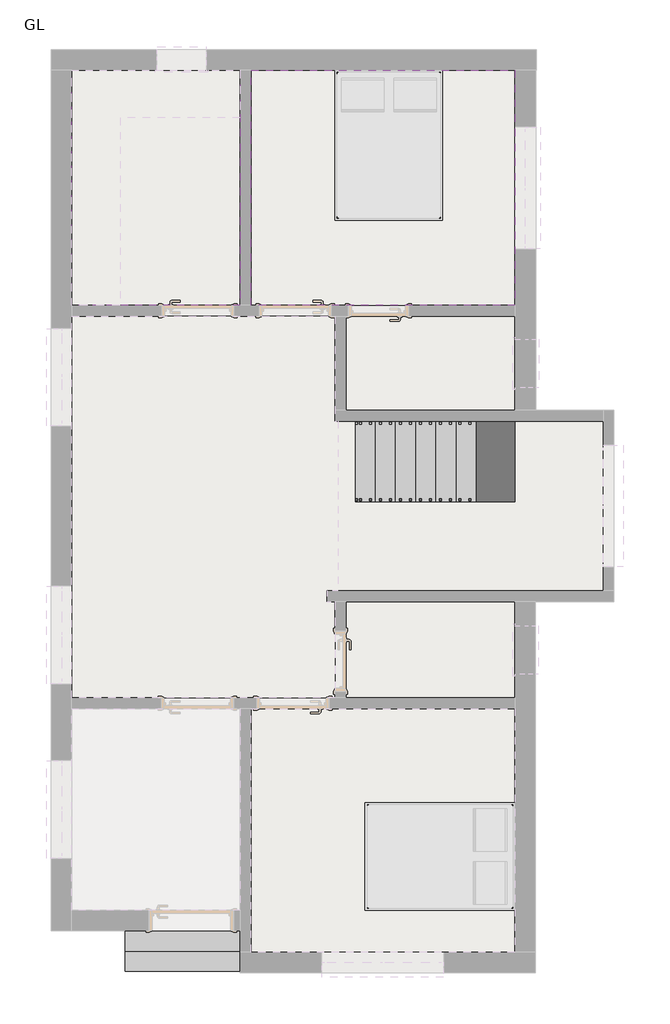
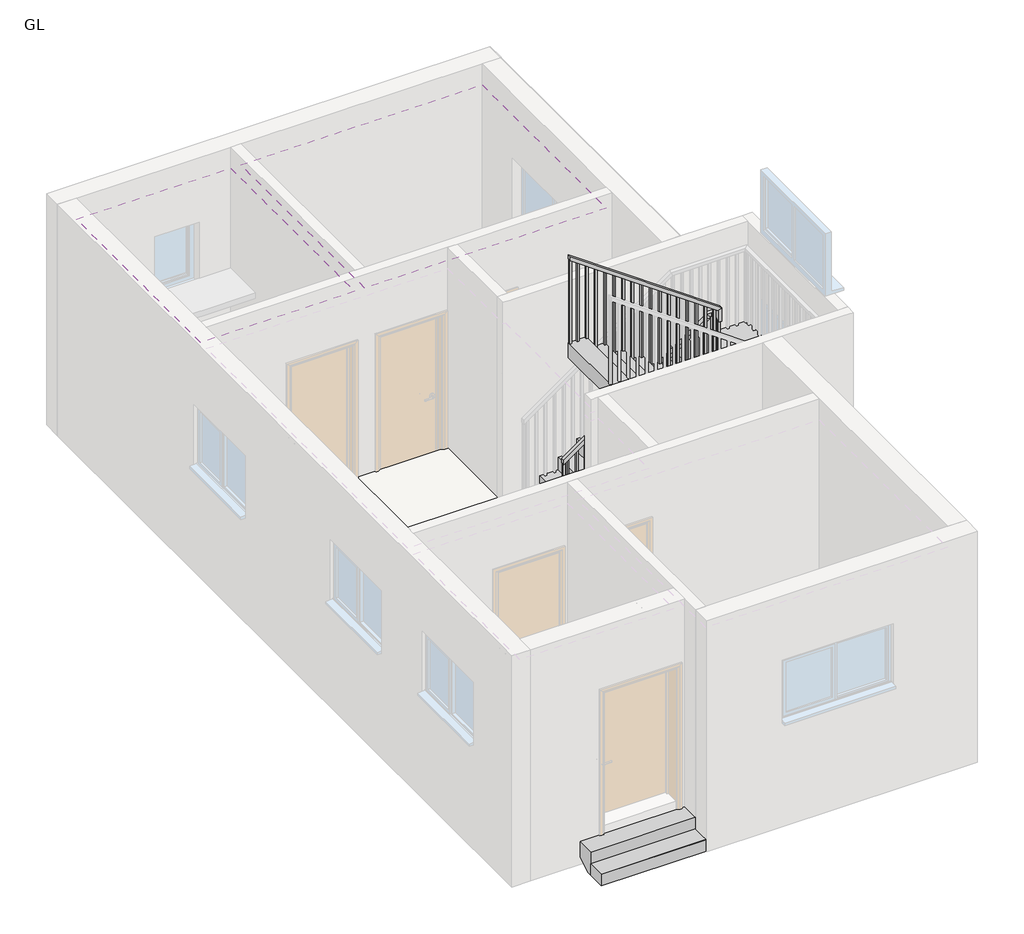
# One storey, part 2 of 3: 4 slabs, 2 coverings, 2 stair flights, 1 railing.
"""IFC4 building model written with IfcOpenShell, lengths in millimetres."""

from ifc_helpers import new_model, si_unit, frame, origin, origin_with_axes, place, context, project, spatial, polyline, outline, extrude, faceted_brep, element, save

model = new_model("IFC4")

# Units and contexts
model_context = context("Model", 3, world=origin())
ifc_project = project(units=[si_unit("LENGTHUNIT", "METRE", prefix="MILLI")], contexts=[model_context])

# Site, building, storey
site = spatial("IfcSite", under=ifc_project)
building = spatial("IfcBuilding", under=site)
storey = spatial("IfcBuildingStorey", under=building, Name="GL", Elevation=0.0)

# Coverings
placement = place(None, origin())
element("IfcCovering", 1, ObjectType="Plain", at=placement, inside=storey, context=model_context, shape_type="SweptSolid", body=[
    extrude(outline(polyline([(-5865.3374044, 11850.4554997), (-3749.5174044, 11850.4554997), (-3749.5174044, 8899.3621562), (-5865.3374044, 8899.3621562), (-5865.3374044, 11850.4554997)])), frame((0.0, 0.0, 2743.2), z_axis=(0.0, 0.0, 1.0), x_axis=(1.0, 0.0, 0.0)), (0.0, 0.0, 1.0), 57.0),
])
element("IfcCovering", 2, ObjectType="Plain", at=placement, inside=storey, context=model_context, shape_type="SweptSolid", body=[
    extrude(outline(polyline([(-3612.3574044, 11850.4554997), (-299.7708818, 11850.4554997), (-299.7708818, 8899.3621562), (-3612.3574044, 8899.3621562), (-3612.3574044, 11850.4554997)])), frame((0.0, 0.0, 2743.2), z_axis=(0.0, 0.0, 1.0), x_axis=(1.0, 0.0, 0.0)), (0.0, 0.0, 1.0), 57.0),
])

# Railing
element("IfcRailing", 3, ObjectType="1100mm", at=placement, inside=storey, context=model_context, shape_type="SolidModel", body=[
    faceted_brep([(-2302.0068409, 6487.2975222, 1279.2941176), (-2302.0068409, 6487.2975222, 1218.028329), (-2302.0068409, 6437.2975222, 1218.028329), (-2302.0068409, 6437.2975222, 1279.2941176), (-350.9568409, 6487.2975222, 2660.8231606), (-300.9568409, 6487.2975222, 2634.9621295), (-300.9568409, 6437.2975222, 2634.9621295), (-350.9568409, 6437.2975222, 2660.8231606), (-350.9568409, 6487.2975222, 2713.6470588), (-300.9568409, 6487.2975222, 2663.6470588), (-300.9568409, 6437.2975222, 2663.6470588), (-350.9568409, 6437.2975222, 2713.6470588), (-225.9568409, 6487.2975222, 2713.6470588), (-225.9568409, 6487.2975222, 2663.6470588), (-275.9568409, 6437.2975222, 2663.6470588), (-275.9568409, 6437.2975222, 2713.6470588), (-225.9568409, 6362.2975222, 2713.6470588), (-225.9568409, 6362.2975222, 2663.6470588), (-275.9568409, 6362.2975222, 2663.6470588), (-275.9568409, 6362.2975222, 2713.6470588), (-225.9568409, 6334.8975222, 2713.6470588), (-275.9568409, 6334.8975222, 2713.6470588), (-275.9568409, 6284.8975222, 2663.6470588), (-225.9568409, 6284.8975222, 2663.6470588)], [[[0, 1, 2, 3]], [[1, 0, 4, 5]], [[2, 1, 5, 6]], [[3, 2, 6, 7]], [[0, 3, 7, 4]], [[5, 4, 8, 9]], [[6, 5, 9, 10]], [[7, 6, 10, 11]], [[4, 7, 11, 8]], [[9, 8, 12, 13]], [[10, 9, 13, 14]], [[11, 10, 14, 15]], [[8, 11, 15, 12]], [[13, 12, 16, 17]], [[14, 13, 17, 18]], [[15, 14, 18, 19]], [[12, 15, 19, 16]], [[20, 21, 22, 23]], [[17, 16, 20, 23]], [[18, 17, 23, 22]], [[19, 18, 22, 21]], [[16, 19, 21, 20]]]),
    faceted_brep([(-225.9568409, 6334.8975222, 2713.6470588), (-225.9568409, 6284.8975222, 2663.6470588), (-275.9568409, 6284.8975222, 2663.6470588), (-275.9568409, 6334.8975222, 2713.6470588), (-225.9568409, 6334.8975222, 2857.2531809), (-275.9568409, 6334.8975222, 2831.3921498), (-275.9568409, 6284.8975222, 2831.3921498), (-225.9568409, 6284.8975222, 2857.2531809)], [[[0, 1, 2, 3]], [[4, 5, 6, 7]], [[1, 0, 4, 7]], [[2, 1, 7, 6]], [[3, 2, 6, 5]], [[0, 3, 5, 4]]]),
    faceted_brep([(-225.9568409, 6284.8975222, 2857.2531809), (-275.9568409, 6284.8975222, 2831.3921498), (-275.9568409, 6334.8975222, 2831.3921498), (-225.9568409, 6334.8975222, 2857.2531809), (-2302.0068409, 6284.8975222, 4327.2941176), (-2302.0068409, 6334.8975222, 4327.2941176), (-2302.0068409, 6334.8975222, 4266.028329), (-2302.0068409, 6284.8975222, 4266.028329)], [[[0, 1, 2, 3]], [[4, 5, 6, 7]], [[1, 0, 4, 7]], [[2, 1, 7, 6]], [[3, 2, 6, 5]], [[0, 3, 5, 4]]]),
    extrude(outline(polyline([(3048.0, -2175.9568409), (4176.7729353, -2175.9568409), (4194.4753141, -2200.9568409), (3048.0, -2200.9568409), (3048.0, -2175.9568409)])), frame((0.0, 6297.3975222, 0.0), z_axis=(0.0, 1.0, 0.0), x_axis=(0.0, 0.0, 1.0)), (0.0, 0.0, 1.0), 25.0),
    extrude(outline(polyline([(3048.0, -2050.9568409), (4088.2610416, -2050.9568409), (4105.9634203, -2075.9568409), (3048.0, -2075.9568409), (3048.0, -2050.9568409)])), frame((0.0, 6297.3975222, 0.0), z_axis=(0.0, 1.0, 0.0), x_axis=(0.0, 0.0, 1.0)), (0.0, 0.0, 1.0), 25.0),
    extrude(outline(polyline([(2868.7058824, -1925.9568409), (3999.7491478, -1925.9568409), (4017.4515265, -1950.9568409), (2868.7058824, -1950.9568409), (2868.7058824, -1925.9568409)])), frame((0.0, 6297.3975222, 0.0), z_axis=(0.0, 1.0, 0.0), x_axis=(0.0, 0.0, 1.0)), (0.0, 0.0, 1.0), 25.0),
    extrude(outline(polyline([(2868.7058824, -1800.9568409), (3911.237254, -1800.9568409), (3928.9396327, -1825.9568409), (2868.7058824, -1825.9568409), (2868.7058824, -1800.9568409)])), frame((0.0, 6297.3975222, 0.0), z_axis=(0.0, 1.0, 0.0), x_axis=(0.0, 0.0, 1.0)), (0.0, 0.0, 1.0), 25.0),
    extrude(outline(polyline([(2689.4117647, -1675.9568409), (3822.7253602, -1675.9568409), (3840.427739, -1700.9568409), (2689.4117647, -1700.9568409), (2689.4117647, -1675.9568409)])), frame((0.0, 6297.3975222, 0.0), z_axis=(0.0, 1.0, 0.0), x_axis=(0.0, 0.0, 1.0)), (0.0, 0.0, 1.0), 25.0),
    extrude(outline(polyline([(2689.4117647, -1550.9568409), (3734.2134664, -1550.9568409), (3751.9158452, -1575.9568409), (2689.4117647, -1575.9568409), (2689.4117647, -1550.9568409)])), frame((0.0, 6297.3975222, 0.0), z_axis=(0.0, 1.0, 0.0), x_axis=(0.0, 0.0, 1.0)), (0.0, 0.0, 1.0), 25.0),
    extrude(outline(polyline([(2510.1176471, -1425.9568409), (3645.7015726, -1425.9568409), (3663.4039514, -1450.9568409), (2510.1176471, -1450.9568409), (2510.1176471, -1425.9568409)])), frame((0.0, 6297.3975222, 0.0), z_axis=(0.0, 1.0, 0.0), x_axis=(0.0, 0.0, 1.0)), (0.0, 0.0, 1.0), 25.0),
    extrude(outline(polyline([(2510.1176471, -1300.9568409), (3557.1896788, -1300.9568409), (3574.8920576, -1325.9568409), (2510.1176471, -1325.9568409), (2510.1176471, -1300.9568409)])), frame((0.0, 6297.3975222, 0.0), z_axis=(0.0, 1.0, 0.0), x_axis=(0.0, 0.0, 1.0)), (0.0, 0.0, 1.0), 25.0),
    extrude(outline(polyline([(2330.8235294, -1175.9568409), (3468.6777851, -1175.9568409), (3486.3801638, -1200.9568409), (2330.8235294, -1200.9568409), (2330.8235294, -1175.9568409)])), frame((0.0, 6297.3975222, 0.0), z_axis=(0.0, 1.0, 0.0), x_axis=(0.0, 0.0, 1.0)), (0.0, 0.0, 1.0), 25.0),
    extrude(outline(polyline([(2330.8235294, -1050.9568409), (3380.1658913, -1050.9568409), (3397.86827, -1075.9568409), (2330.8235294, -1075.9568409), (2330.8235294, -1050.9568409)])), frame((0.0, 6297.3975222, 0.0), z_axis=(0.0, 1.0, 0.0), x_axis=(0.0, 0.0, 1.0)), (0.0, 0.0, 1.0), 25.0),
    extrude(outline(polyline([(2151.5294118, -925.9568409), (3291.6539975, -925.9568409), (3309.3563762, -950.9568409), (2151.5294118, -950.9568409), (2151.5294118, -925.9568409)])), frame((0.0, 6297.3975222, 0.0), z_axis=(0.0, 1.0, 0.0), x_axis=(0.0, 0.0, 1.0)), (0.0, 0.0, 1.0), 25.0),
    extrude(outline(polyline([(2151.5294118, -800.9568409), (3203.1421037, -800.9568409), (3220.8444825, -825.9568409), (2151.5294118, -825.9568409), (2151.5294118, -800.9568409)])), frame((0.0, 6297.3975222, 0.0), z_axis=(0.0, 1.0, 0.0), x_axis=(0.0, 0.0, 1.0)), (0.0, 0.0, 1.0), 25.0),
    extrude(outline(polyline([(1972.2352941, -675.9568409), (3114.6302099, -675.9568409), (3132.3325887, -700.9568409), (1972.2352941, -700.9568409), (1972.2352941, -675.9568409)])), frame((0.0, 6297.3975222, 0.0), z_axis=(0.0, 1.0, 0.0), x_axis=(0.0, 0.0, 1.0)), (0.0, 0.0, 1.0), 25.0),
    extrude(outline(polyline([(1972.2352941, -550.9568409), (3026.1183161, -550.9568409), (3043.8206949, -575.9568409), (1972.2352941, -575.9568409), (1972.2352941, -550.9568409)])), frame((0.0, 6297.3975222, 0.0), z_axis=(0.0, 1.0, 0.0), x_axis=(0.0, 0.0, 1.0)), (0.0, 0.0, 1.0), 25.0),
    extrude(outline(polyline([(1792.9411765, -425.9568409), (2937.6064223, -425.9568409), (2955.3088011, -450.9568409), (1792.9411765, -450.9568409), (1792.9411765, -425.9568409)])), frame((0.0, 6297.3975222, 0.0), z_axis=(0.0, 1.0, 0.0), x_axis=(0.0, 0.0, 1.0)), (0.0, 0.0, 1.0), 25.0),
    extrude(outline(polyline([(1792.9411765, -300.9568409), (2849.0945286, -300.9568409), (2866.7969073, -325.9568409), (1792.9411765, -325.9568409), (1792.9411765, -300.9568409)])), frame((0.0, 6297.3975222, 0.0), z_axis=(0.0, 1.0, 0.0), x_axis=(0.0, 0.0, 1.0)), (0.0, 0.0, 1.0), 25.0),
    extrude(outline(polyline([(-263.4568409, 6412.2975222), (-238.4568409, 6412.2975222), (-238.4568409, 6387.2975222), (-263.4568409, 6387.2975222), (-263.4568409, 6412.2975222)])), frame((0.0, 0.0, 1613.6470588), z_axis=(0.0, 0.0, 1.0), x_axis=(1.0, 0.0, 0.0)), (0.0, 0.0, 1.0), 1050.0),
    extrude(outline(polyline([(2581.1114933, -377.0068409), (1434.3529412, -377.0068409), (1434.3529412, -352.0068409), (2598.8138721, -352.0068409), (2581.1114933, -377.0068409)])), frame((0.0, 6449.7975222, 0.0), z_axis=(0.0, 1.0, 0.0), x_axis=(0.0, 0.0, 1.0)), (0.0, 0.0, 1.0), 25.0),
    extrude(outline(polyline([(2492.5995995, -502.0068409), (1434.3529412, -502.0068409), (1434.3529412, -477.0068409), (2510.3019783, -477.0068409), (2492.5995995, -502.0068409)])), frame((0.0, 6449.7975222, 0.0), z_axis=(0.0, 1.0, 0.0), x_axis=(0.0, 0.0, 1.0)), (0.0, 0.0, 1.0), 25.0),
    extrude(outline(polyline([(2404.0877058, -627.0068409), (1255.0588235, -627.0068409), (1255.0588235, -602.0068409), (2421.7900845, -602.0068409), (2404.0877058, -627.0068409)])), frame((0.0, 6449.7975222, 0.0), z_axis=(0.0, 1.0, 0.0), x_axis=(0.0, 0.0, 1.0)), (0.0, 0.0, 1.0), 25.0),
    extrude(outline(polyline([(2315.575812, -752.0068409), (1255.0588235, -752.0068409), (1255.0588235, -727.0068409), (2333.2781907, -727.0068409), (2315.575812, -752.0068409)])), frame((0.0, 6449.7975222, 0.0), z_axis=(0.0, 1.0, 0.0), x_axis=(0.0, 0.0, 1.0)), (0.0, 0.0, 1.0), 25.0),
    extrude(outline(polyline([(2227.0639182, -877.0068409), (1075.7647059, -877.0068409), (1075.7647059, -852.0068409), (2244.7662969, -852.0068409), (2227.0639182, -877.0068409)])), frame((0.0, 6449.7975222, 0.0), z_axis=(0.0, 1.0, 0.0), x_axis=(0.0, 0.0, 1.0)), (0.0, 0.0, 1.0), 25.0),
    extrude(outline(polyline([(2138.5520244, -1002.0068409), (1075.7647059, -1002.0068409), (1075.7647059, -977.0068409), (2156.2544032, -977.0068409), (2138.5520244, -1002.0068409)])), frame((0.0, 6449.7975222, 0.0), z_axis=(0.0, 1.0, 0.0), x_axis=(0.0, 0.0, 1.0)), (0.0, 0.0, 1.0), 25.0),
    extrude(outline(polyline([(2050.0401306, -1127.0068409), (896.4705882, -1127.0068409), (896.4705882, -1102.0068409), (2067.7425094, -1102.0068409), (2050.0401306, -1127.0068409)])), frame((0.0, 6449.7975222, 0.0), z_axis=(0.0, 1.0, 0.0), x_axis=(0.0, 0.0, 1.0)), (0.0, 0.0, 1.0), 25.0),
    extrude(outline(polyline([(1961.5282368, -1252.0068409), (896.4705882, -1252.0068409), (896.4705882, -1227.0068409), (1979.2306156, -1227.0068409), (1961.5282368, -1252.0068409)])), frame((0.0, 6449.7975222, 0.0), z_axis=(0.0, 1.0, 0.0), x_axis=(0.0, 0.0, 1.0)), (0.0, 0.0, 1.0), 25.0),
    extrude(outline(polyline([(1873.016343, -1377.0068409), (717.1764706, -1377.0068409), (717.1764706, -1352.0068409), (1890.7187218, -1352.0068409), (1873.016343, -1377.0068409)])), frame((0.0, 6449.7975222, 0.0), z_axis=(0.0, 1.0, 0.0), x_axis=(0.0, 0.0, 1.0)), (0.0, 0.0, 1.0), 25.0),
    extrude(outline(polyline([(1784.5044493, -1502.0068409), (717.1764706, -1502.0068409), (717.1764706, -1477.0068409), (1802.206828, -1477.0068409), (1784.5044493, -1502.0068409)])), frame((0.0, 6449.7975222, 0.0), z_axis=(0.0, 1.0, 0.0), x_axis=(0.0, 0.0, 1.0)), (0.0, 0.0, 1.0), 25.0),
    extrude(outline(polyline([(1695.9925555, -1627.0068409), (537.8823529, -1627.0068409), (537.8823529, -1602.0068409), (1713.6949342, -1602.0068409), (1695.9925555, -1627.0068409)])), frame((0.0, 6449.7975222, 0.0), z_axis=(0.0, 1.0, 0.0), x_axis=(0.0, 0.0, 1.0)), (0.0, 0.0, 1.0), 25.0),
    extrude(outline(polyline([(1607.4806617, -1752.0068409), (537.8823529, -1752.0068409), (537.8823529, -1727.0068409), (1625.1830404, -1727.0068409), (1607.4806617, -1752.0068409)])), frame((0.0, 6449.7975222, 0.0), z_axis=(0.0, 1.0, 0.0), x_axis=(0.0, 0.0, 1.0)), (0.0, 0.0, 1.0), 25.0),
    extrude(outline(polyline([(1518.9687679, -1877.0068409), (358.5882353, -1877.0068409), (358.5882353, -1852.0068409), (1536.6711467, -1852.0068409), (1518.9687679, -1877.0068409)])), frame((0.0, 6449.7975222, 0.0), z_axis=(0.0, 1.0, 0.0), x_axis=(0.0, 0.0, 1.0)), (0.0, 0.0, 1.0), 25.0),
    extrude(outline(polyline([(1430.4568741, -2002.0068409), (358.5882353, -2002.0068409), (358.5882353, -1977.0068409), (1448.1592529, -1977.0068409), (1430.4568741, -2002.0068409)])), frame((0.0, 6449.7975222, 0.0), z_axis=(0.0, 1.0, 0.0), x_axis=(0.0, 0.0, 1.0)), (0.0, 0.0, 1.0), 25.0),
    extrude(outline(polyline([(1341.9449803, -2127.0068409), (179.2941176, -2127.0068409), (179.2941176, -2102.0068409), (1359.6473591, -2102.0068409), (1341.9449803, -2127.0068409)])), frame((0.0, 6449.7975222, 0.0), z_axis=(0.0, 1.0, 0.0), x_axis=(0.0, 0.0, 1.0)), (0.0, 0.0, 1.0), 25.0),
    extrude(outline(polyline([(1253.4330865, -2252.0068409), (179.2941176, -2252.0068409), (179.2941176, -2227.0068409), (1271.1354653, -2227.0068409), (1253.4330865, -2252.0068409)])), frame((0.0, 6449.7975222, 0.0), z_axis=(0.0, 1.0, 0.0), x_axis=(0.0, 0.0, 1.0)), (0.0, 0.0, 1.0), 25.0),
    extrude(outline(polyline([(-263.4568409, 6322.3975222), (-238.4568409, 6322.3975222), (-238.4568409, 6297.3975222), (-263.4568409, 6297.3975222), (-263.4568409, 6322.3975222)])), frame((0.0, 0.0, 1613.6470588), z_axis=(0.0, 0.0, 1.0), x_axis=(1.0, 0.0, 0.0)), (0.0, 0.0, 1.0), 1050.0),
    extrude(outline(polyline([(-263.4568409, 6449.7975222), (-263.4568409, 6474.7975222), (-238.4568409, 6474.7975222), (-238.4568409, 6449.7975222), (-263.4568409, 6449.7975222)])), frame((0.0, 0.0, 1613.6470588), z_axis=(0.0, 0.0, 1.0), x_axis=(1.0, 0.0, 0.0)), (0.0, 0.0, 1.0), 1050.0),
    extrude(outline(polyline([(3048.0, -2277.0068409), (4248.3259503, -2277.0068409), (4266.028329, -2302.0068409), (3048.0, -2302.0068409), (3048.0, -2277.0068409)])), frame((0.0, 6297.3975222, 0.0), z_axis=(0.0, 1.0, 0.0), x_axis=(0.0, 0.0, 1.0)), (0.0, 0.0, 1.0), 25.0),
    extrude(outline(polyline([(1218.028329, -2302.0068409), (179.2941176, -2302.0068409), (179.2941176, -2277.0068409), (1235.7307078, -2277.0068409), (1218.028329, -2302.0068409)])), frame((0.0, 6449.7975222, 0.0), z_axis=(0.0, 1.0, 0.0), x_axis=(0.0, 0.0, 1.0)), (0.0, 0.0, 1.0), 25.0),
])

# Slabs
element("IfcSlab", 4, ObjectType="BEDROOM FLOOR", at=placement, inside=storey, context=model_context, shape_type="SweptSolid", body=[
    extrude(outline(polyline([(-299.7708818, 11850.4554997), (-299.7708818, 8899.3621562), (-3612.3574044, 8899.3621562), (-3612.3574044, 11850.4554997), (-299.7708818, 11850.4554997)])), origin_with_axes(), (0.0, 0.0, 1.0), 149.9616),
    extrude(outline(polyline([(-301.4674044, 3840.8703577), (-301.4674044, 786.2154997), (-3617.4374044, 786.2154997), (-3617.4374044, 3840.8703577), (-301.4674044, 3840.8703577)])), origin_with_axes(), (0.0, 0.0, 1.0), 149.9616),
])
element("IfcSlab", 5, ObjectType="HALL FLOOR", at=placement, inside=storey, context=model_context, shape_type="SweptSolid", body=[
    extrude(outline(polyline([(-2558.2574044, 8762.2021562), (-2558.2574044, 7446.2287671), (804.5291182, 7446.2287671), (804.5291182, 5317.8803577), (-2560.7974044, 5317.8803577), (-2560.7974044, 3978.0303577), (-5865.3374044, 3978.0303577), (-5865.3374044, 8762.2021562), (-2558.2574044, 8762.2021562)])), origin_with_axes(), (0.0, 0.0, 1.0), 149.9616),
])
element("IfcSlab", 6, ObjectType="KITCHEN FLOOR", at=placement, inside=storey, context=model_context, shape_type="SweptSolid", body=[
    extrude(outline(polyline([(-3749.5174044, 11850.4554997), (-3749.5174044, 8899.3621562), (-5865.3374044, 8899.3621562), (-5865.3374044, 11850.4554997), (-3749.5174044, 11850.4554997)])), origin_with_axes(), (0.0, 0.0, 1.0), 149.9616),
])
element("IfcSlab", 7, ObjectType="TOILET", at=placement, inside=storey, context=model_context, shape_type="SweptSolid", body=[
    extrude(outline(polyline([(-2423.6374044, 3978.0303577), (-2423.6374044, 5180.7203577), (-301.4674044, 5180.7203577), (-301.4674044, 3978.0303577), (-2423.6374044, 3978.0303577)])), origin_with_axes(), (0.0, 0.0, 1.0), 149.9616),
    extrude(outline(polyline([(-2421.0974044, 7583.3887671), (-2421.0974044, 8762.2021562), (-299.7708818, 8762.2021562), (-299.7708818, 7583.3887671), (-2421.0974044, 7583.3887671)])), origin_with_axes(), (0.0, 0.0, 1.0), 149.9616),
])

# Stair flights
element("IfcStairFlight", 8, ObjectType="1mm_Tread-175mm_Depth", at=placement, inside=storey, context=model_context, shape_type="SolidModel", body=[
    faceted_brep([(-2054.3568409, 7446.2287671, 178.2941176), (-2302.0068409, 7446.2287671, 178.2941176), (-2302.0068409, 6436.8975222, 178.2941176), (-2054.3568409, 6436.8975222, 178.2941176), (-2054.3568409, 7446.2287671, 3.2941176), (-2302.0068409, 7446.2287671, 3.2941176), (-2302.0068409, 6436.8975222, 3.2941176), (-2054.3568409, 6436.8975222, 3.2941176), (-2054.3568409, 7446.2287671, 357.5882353), (-2054.3568409, 6436.8975222, 357.5882353), (-1998.8139986, 6436.8975222, 357.5882353), (-1800.3568409, 6436.8975222, 357.5882353), (-1800.3568409, 7446.2287671, 357.5882353), (-1998.8139986, 7446.2287671, 357.5882353), (-1800.3568409, 7446.2287671, 143.381523), (-1998.8139986, 7446.2287671, 3.2941176), (-1998.8139986, 6436.8975222, 3.2941176), (-1800.3568409, 6436.8975222, 143.381523), (-1546.3568409, 7446.2287671, 536.8823529), (-1800.3568409, 7446.2287671, 536.8823529), (-1800.3568409, 6436.8975222, 536.8823529), (-1546.3568409, 6436.8975222, 536.8823529), (-1546.3568409, 7446.2287671, 322.6756407), (-1546.3568409, 6436.8975222, 322.6756407), (-1292.3568409, 7446.2287671, 716.1764706), (-1546.3568409, 7446.2287671, 716.1764706), (-1546.3568409, 6436.8975222, 716.1764706), (-1292.3568409, 6436.8975222, 716.1764706), (-1292.3568409, 7446.2287671, 501.9697583), (-1292.3568409, 6436.8975222, 501.9697583), (-1038.3568409, 7446.2287671, 895.4705882), (-1292.3568409, 7446.2287671, 895.4705882), (-1292.3568409, 6436.8975222, 895.4705882), (-1038.3568409, 6436.8975222, 895.4705882), (-1038.3568409, 7446.2287671, 681.263876), (-1038.3568409, 6436.8975222, 681.263876), (-784.3568409, 7446.2287671, 1074.7647059), (-1038.3568409, 7446.2287671, 1074.7647059), (-1038.3568409, 6436.8975222, 1074.7647059), (-784.3568409, 6436.8975222, 1074.7647059), (-784.3568409, 7446.2287671, 860.5579936), (-784.3568409, 6436.8975222, 860.5579936), (-530.3568409, 7446.2287671, 1254.0588235), (-784.3568409, 7446.2287671, 1254.0588235), (-784.3568409, 6436.8975222, 1254.0588235), (-530.3568409, 6436.8975222, 1254.0588235), (-530.3568409, 7446.2287671, 1039.8521113), (-530.3568409, 6436.8975222, 1039.8521113), (-276.3568409, 7446.2287671, 1433.3529412), (-530.3568409, 7446.2287671, 1433.3529412), (-530.3568409, 6436.8975222, 1433.3529412), (-276.3568409, 6436.8975222, 1433.3529412), (-276.3568409, 7446.2287671, 1219.1462289), (33.1860014, 6436.8975222, 1437.6470588), (-276.3568409, 6436.8975222, 1437.6470588), (-276.3568409, 5317.8803577, 1612.6470588), (788.0478774, 5317.8803577, 1612.6470588), (788.0478774, 7446.2287671, 1612.6470588), (33.1860014, 7446.2287671, 1612.6470588), (-276.3568409, 7446.2287671, 1612.6470588), (-276.3568409, 6436.8975222, 1612.6470588), (-276.3568409, 6335.2975222, 1612.6470588), (-276.3568409, 5317.8803577, 1437.6470588), (788.0478774, 5317.8803577, 1437.6470588), (788.0478774, 7446.2287671, 1437.6470588), (33.1860014, 7446.2287671, 1437.6470588), (-276.3568409, 6335.2975222, 1437.6470588), (-276.3568409, 5317.8803577, 1791.9411765), (-276.3568409, 6335.2975222, 1791.9411765), (-331.8996832, 6335.2975222, 1791.9411765), (-536.5621226, 6335.2975222, 1791.9411765), (-536.5621226, 5317.8803577, 1791.9411765), (-331.8996832, 5317.8803577, 1791.9411765), (-536.5621226, 5317.8803577, 1582.1146631), (-331.8996832, 5317.8803577, 1437.6470588), (-331.8996832, 6335.2975222, 1437.6470588), (-536.5621226, 6335.2975222, 1582.1146631), (-790.5621226, 5317.8803577, 1971.2352941), (-536.5621226, 5317.8803577, 1971.2352941), (-536.5621226, 6335.2975222, 1971.2352941), (-790.5621226, 6335.2975222, 1971.2352941), (-790.5621226, 5317.8803577, 1761.4087807), (-790.5621226, 6335.2975222, 1761.4087807), (-1044.5621226, 5317.8803577, 2150.5294118), (-790.5621226, 5317.8803577, 2150.5294118), (-790.5621226, 6335.2975222, 2150.5294118), (-1044.5621226, 6335.2975222, 2150.5294118), (-1044.5621226, 5317.8803577, 1940.7028984), (-1044.5621226, 6335.2975222, 1940.7028984), (-1289.1818409, 5317.8803577, 2329.8235294), (-1044.5621226, 5317.8803577, 2329.8235294), (-1044.5621226, 6335.2975222, 2329.8235294), (-1289.1818409, 6335.2975222, 2329.8235294), (-1289.1818409, 5317.8803577, 2113.3756407), (-1289.1818409, 6335.2975222, 2113.3756407), (-1546.3568409, 5317.8803577, 2509.1176471), (-1289.1818409, 5317.8803577, 2509.1176471), (-1289.1818409, 6335.2975222, 2509.1176471), (-1546.3568409, 6335.2975222, 2509.1176471), (-1546.3568409, 5317.8803577, 2294.9109348), (-1546.3568409, 6335.2975222, 2294.9109348), (-1800.3568409, 5317.8803577, 2688.4117647), (-1546.3568409, 5317.8803577, 2688.4117647), (-1546.3568409, 6335.2975222, 2688.4117647), (-1800.3568409, 6335.2975222, 2688.4117647), (-1800.3568409, 5317.8803577, 2474.2050525), (-1800.3568409, 6335.2975222, 2474.2050525), (-2054.3568409, 5317.8803577, 2867.7058824), (-1800.3568409, 5317.8803577, 2867.7058824), (-1800.3568409, 6335.2975222, 2867.7058824), (-2054.3568409, 6335.2975222, 2867.7058824), (-2054.3568409, 5317.8803577, 2653.4991701), (-2054.3568409, 6335.2975222, 2653.4991701), (-2302.0068409, 5317.8803577, 3047.0), (-2054.3568409, 5317.8803577, 3047.0), (-2054.3568409, 6335.2975222, 3047.0), (-2302.0068409, 6335.2975222, 3047.0), (-2302.0068409, 5317.8803577, 2828.3109348), (-2302.0068409, 6335.2975222, 2828.3109348)], [[[0, 1, 2, 3]], [[1, 0, 4, 5]], [[2, 1, 5, 6]], [[3, 2, 6, 7]], [[8, 9, 10, 11, 12, 13]], [[0, 8, 13, 12, 14, 15, 4]], [[0, 3, 9, 8]], [[9, 3, 7, 16, 17, 11, 10]], [[18, 19, 20, 21]], [[19, 18, 22, 14, 12]], [[12, 11, 20, 19]], [[21, 20, 11, 17, 23]], [[24, 25, 26, 27]], [[25, 24, 28, 22, 18]], [[18, 21, 26, 25]], [[27, 26, 21, 23, 29]], [[30, 31, 32, 33]], [[31, 30, 34, 28, 24]], [[24, 27, 32, 31]], [[33, 32, 27, 29, 35]], [[36, 37, 38, 39]], [[37, 36, 40, 34, 30]], [[30, 33, 38, 37]], [[39, 38, 33, 35, 41]], [[42, 43, 44, 45]], [[43, 42, 46, 40, 36]], [[36, 39, 44, 43]], [[45, 44, 39, 41, 47]], [[48, 49, 50, 51]], [[49, 48, 52, 46, 42]], [[42, 45, 50, 49]], [[51, 50, 45, 47, 53, 54]], [[55, 56, 57, 58, 59, 60, 61]], [[56, 55, 62, 63]], [[57, 56, 63, 64]], [[48, 59, 58, 57, 64, 65, 52]], [[48, 51, 54, 60, 59]], [[61, 60, 54, 66]], [[67, 68, 69, 70, 71, 72]], [[55, 67, 72, 71, 73, 74, 62]], [[55, 61, 68, 67]], [[68, 61, 66, 75, 76, 70, 69]], [[77, 78, 79, 80]], [[78, 77, 81, 73, 71]], [[71, 70, 79, 78]], [[80, 79, 70, 76, 82]], [[83, 84, 85, 86]], [[84, 83, 87, 81, 77]], [[77, 80, 85, 84]], [[86, 85, 80, 82, 88]], [[89, 90, 91, 92]], [[90, 89, 93, 87, 83]], [[83, 86, 91, 90]], [[92, 91, 86, 88, 94]], [[95, 96, 97, 98]], [[96, 95, 99, 93, 89]], [[89, 92, 97, 96]], [[98, 97, 92, 94, 100]], [[101, 102, 103, 104]], [[102, 101, 105, 99, 95]], [[95, 98, 103, 102]], [[104, 103, 98, 100, 106]], [[107, 108, 109, 110]], [[108, 107, 111, 105, 101]], [[101, 104, 109, 108]], [[110, 109, 104, 106, 112]], [[113, 114, 115, 116]], [[114, 113, 117, 111, 107]], [[107, 110, 115, 114]], [[116, 115, 110, 112, 118]], [[113, 116, 118, 117]], [[15, 16, 7, 6, 5, 4]], [[16, 15, 14, 22, 28, 34, 40, 46, 52, 65, 53, 47, 41, 35, 29, 23, 17]], [[53, 65, 64, 63, 62, 74, 75, 66, 54]], [[75, 74, 73, 81, 87, 93, 99, 105, 111, 117, 118, 112, 106, 100, 94, 88, 82, 76]]]),
    extrude(outline(polyline([(-2054.3568409, 7446.2287671), (-2054.3568409, 6436.8975222), (-2302.0068409, 6436.8975222), (-2302.0068409, 7446.2287671), (-2054.3568409, 7446.2287671)])), frame((0.0, 0.0, 178.2941176), z_axis=(0.0, 0.0, 1.0), x_axis=(1.0, 0.0, 0.0)), (0.0, 0.0, 1.0), 1.0),
    extrude(outline(polyline([(-1800.3568409, 7446.2287671), (-1800.3568409, 6436.8975222), (-2054.3568409, 6436.8975222), (-2054.3568409, 7446.2287671), (-1800.3568409, 7446.2287671)])), frame((0.0, 0.0, 357.5882353), z_axis=(0.0, 0.0, 1.0), x_axis=(1.0, 0.0, 0.0)), (0.0, 0.0, 1.0), 1.0),
    extrude(outline(polyline([(-1546.3568409, 7446.2287671), (-1546.3568409, 6436.8975222), (-1800.3568409, 6436.8975222), (-1800.3568409, 7446.2287671), (-1546.3568409, 7446.2287671)])), frame((0.0, 0.0, 536.8823529), z_axis=(0.0, 0.0, 1.0), x_axis=(1.0, 0.0, 0.0)), (0.0, 0.0, 1.0), 1.0),
    extrude(outline(polyline([(-1292.3568409, 7446.2287671), (-1292.3568409, 6436.8975222), (-1546.3568409, 6436.8975222), (-1546.3568409, 7446.2287671), (-1292.3568409, 7446.2287671)])), frame((0.0, 0.0, 716.1764706), z_axis=(0.0, 0.0, 1.0), x_axis=(1.0, 0.0, 0.0)), (0.0, 0.0, 1.0), 1.0),
    extrude(outline(polyline([(-1038.3568409, 7446.2287671), (-1038.3568409, 6436.8975222), (-1292.3568409, 6436.8975222), (-1292.3568409, 7446.2287671), (-1038.3568409, 7446.2287671)])), frame((0.0, 0.0, 895.4705882), z_axis=(0.0, 0.0, 1.0), x_axis=(1.0, 0.0, 0.0)), (0.0, 0.0, 1.0), 1.0),
    extrude(outline(polyline([(-784.3568409, 7446.2287671), (-784.3568409, 6436.8975222), (-1038.3568409, 6436.8975222), (-1038.3568409, 7446.2287671), (-784.3568409, 7446.2287671)])), frame((0.0, 0.0, 1074.7647059), z_axis=(0.0, 0.0, 1.0), x_axis=(1.0, 0.0, 0.0)), (0.0, 0.0, 1.0), 1.0),
    extrude(outline(polyline([(-530.3568409, 7446.2287671), (-530.3568409, 6436.8975222), (-784.3568409, 6436.8975222), (-784.3568409, 7446.2287671), (-530.3568409, 7446.2287671)])), frame((0.0, 0.0, 1254.0588235), z_axis=(0.0, 0.0, 1.0), x_axis=(1.0, 0.0, 0.0)), (0.0, 0.0, 1.0), 1.0),
    extrude(outline(polyline([(-276.3568409, 7446.2287671), (-276.3568409, 6436.8975222), (-530.3568409, 6436.8975222), (-530.3568409, 7446.2287671), (-276.3568409, 7446.2287671)])), frame((0.0, 0.0, 1433.3529412), z_axis=(0.0, 0.0, 1.0), x_axis=(1.0, 0.0, 0.0)), (0.0, 0.0, 1.0), 1.0),
    extrude(outline(polyline([(-276.3568409, 5317.8803577), (-276.3568409, 6335.2975222), (-276.3568409, 6436.8975222), (-276.3568409, 7446.2287671), (788.0478774, 7446.2287671), (788.0478774, 5317.8803577), (-276.3568409, 5317.8803577)])), frame((0.0, 0.0, 1612.6470588), z_axis=(0.0, 0.0, 1.0), x_axis=(1.0, 0.0, 0.0)), (0.0, 0.0, 1.0), 1.0),
    extrude(outline(polyline([(-536.5621226, 5317.8803577), (-536.5621226, 6335.2975222), (-276.3568409, 6335.2975222), (-276.3568409, 5317.8803577), (-536.5621226, 5317.8803577)])), frame((0.0, 0.0, 1791.9411765), z_axis=(0.0, 0.0, 1.0), x_axis=(1.0, 0.0, 0.0)), (0.0, 0.0, 1.0), 1.0),
    extrude(outline(polyline([(-790.5621226, 5317.8803577), (-790.5621226, 6335.2975222), (-536.5621226, 6335.2975222), (-536.5621226, 5317.8803577), (-790.5621226, 5317.8803577)])), frame((0.0, 0.0, 1971.2352941), z_axis=(0.0, 0.0, 1.0), x_axis=(1.0, 0.0, 0.0)), (0.0, 0.0, 1.0), 1.0),
    extrude(outline(polyline([(-1044.5621226, 5317.8803577), (-1044.5621226, 6335.2975222), (-790.5621226, 6335.2975222), (-790.5621226, 5317.8803577), (-1044.5621226, 5317.8803577)])), frame((0.0, 0.0, 2150.5294118), z_axis=(0.0, 0.0, 1.0), x_axis=(1.0, 0.0, 0.0)), (0.0, 0.0, 1.0), 1.0),
    extrude(outline(polyline([(-1289.1818409, 5317.8803577), (-1289.1818409, 6335.2975222), (-1044.5621226, 6335.2975222), (-1044.5621226, 5317.8803577), (-1289.1818409, 5317.8803577)])), frame((0.0, 0.0, 2329.8235294), z_axis=(0.0, 0.0, 1.0), x_axis=(1.0, 0.0, 0.0)), (0.0, 0.0, 1.0), 1.0),
    extrude(outline(polyline([(-1546.3568409, 5317.8803577), (-1546.3568409, 6335.2975222), (-1289.1818409, 6335.2975222), (-1289.1818409, 5317.8803577), (-1546.3568409, 5317.8803577)])), frame((0.0, 0.0, 2509.1176471), z_axis=(0.0, 0.0, 1.0), x_axis=(1.0, 0.0, 0.0)), (0.0, 0.0, 1.0), 1.0),
    extrude(outline(polyline([(-1800.3568409, 5317.8803577), (-1800.3568409, 6335.2975222), (-1546.3568409, 6335.2975222), (-1546.3568409, 5317.8803577), (-1800.3568409, 5317.8803577)])), frame((0.0, 0.0, 2688.4117647), z_axis=(0.0, 0.0, 1.0), x_axis=(1.0, 0.0, 0.0)), (0.0, 0.0, 1.0), 1.0),
    extrude(outline(polyline([(-2054.3568409, 5317.8803577), (-2054.3568409, 6335.2975222), (-1800.3568409, 6335.2975222), (-1800.3568409, 5317.8803577), (-2054.3568409, 5317.8803577)])), frame((0.0, 0.0, 2867.7058824), z_axis=(0.0, 0.0, 1.0), x_axis=(1.0, 0.0, 0.0)), (0.0, 0.0, 1.0), 1.0),
    extrude(outline(polyline([(-2302.0068409, 5317.8803577), (-2302.0068409, 6335.2975222), (-2054.3568409, 6335.2975222), (-2054.3568409, 5317.8803577), (-2302.0068409, 5317.8803577)])), frame((0.0, 0.0, 3047.0), z_axis=(0.0, 0.0, 1.0), x_axis=(1.0, 0.0, 0.0)), (0.0, 0.0, 1.0), 1.0),
])
element("IfcStairFlight", 9, ObjectType="1mm_Tread-175mm_Depth", at=placement, inside=storey, context=model_context, shape_type="SolidModel", body=[
    faceted_brep([(-5192.2374044, 800.4903577, -138.16), (-5192.2374044, 546.4903577, -138.16), (-3754.5974044, 546.4903577, -138.16), (-3754.5974044, 800.4903577, -138.16), (-5192.2374044, 800.4903577, -304.8), (-5192.2374044, 546.4903577, -304.8), (-3754.5974044, 546.4903577, -304.8), (-3754.5974044, 800.4903577, -304.8), (-5192.2374044, 1054.4903577, 29.48), (-5192.2374044, 800.4903577, 29.48), (-3754.5974044, 800.4903577, 29.48), (-3754.5974044, 1054.4903577, 29.48), (-5192.2374044, 1054.4903577, -180.1989212), (-5192.2374044, 865.7008444, -304.8), (-3754.5974044, 865.7008444, -304.8), (-3754.5974044, 1054.4903577, -180.1989212)], [[[0, 1, 2, 3]], [[1, 0, 4, 5]], [[2, 1, 5, 6]], [[3, 2, 6, 7]], [[8, 9, 10, 11]], [[4, 0, 9, 8, 12, 13]], [[0, 3, 10, 9]], [[3, 7, 14, 15, 11, 10]], [[8, 11, 15, 12]], [[5, 4, 13, 14, 7, 6]], [[14, 13, 12, 15]]]),
    extrude(outline(polyline([(-5192.2374044, 800.4903577), (-3754.5974044, 800.4903577), (-3754.5974044, 546.4903577), (-5192.2374044, 546.4903577), (-5192.2374044, 800.4903577)])), frame((0.0, 0.0, -138.16), z_axis=(0.0, 0.0, 1.0), x_axis=(1.0, 0.0, 0.0)), (0.0, 0.0, 1.0), 1.0),
    extrude(outline(polyline([(-5192.2374044, 1054.4903577), (-3754.5974044, 1054.4903577), (-3754.5974044, 800.4903577), (-5192.2374044, 800.4903577), (-5192.2374044, 1054.4903577)])), frame((0.0, 0.0, 29.48), z_axis=(0.0, 0.0, 1.0), x_axis=(1.0, 0.0, 0.0)), (0.0, 0.0, 1.0), 1.0),
])

save(model, "model.ifc")

# Revit data of these elements
# Type "Plain"
#   Keynote = "K40"
#   built-in parameter 1002203 = 1 (stored number, unit not read)
#   built-in parameter 1002202 = 1 (stored number, unit not read)
#   Layers, outside or top first: 45 mm "Metal Stud Layer" (function 1); 12 mm "Gypsum Wall Board" (function 1)
# Type "1100mm"
#   built-in parameter 1008612 = 0.019685 (stored number, unit not read)
#   built-in parameter 1008611 = 0.019685 (stored number, unit not read)
#   built-in parameter 1008609 = 0.902231 (stored number, unit not read)
#   built-in parameter 1008604 = 0.19685 (stored number, unit not read)
#   built-in parameter 1008603 = 0.164042 (stored number, unit not read)
#   Railing Height = 1100 mm
#   built-in parameter 1008630 = 2
#   built-in parameter 1008610 = 2
#   built-in parameter 1008608 = 1
#   built-in parameter 1008618 = Baluster_Square : 25mm
# Type "BEDROOM FLOOR"
#   Function = 0
#   Layers, outside or top first: 21.946 mm "Wood Sheathing, Chipboard" (function 5); 128.016 mm "Structure, Timber Joist/Rafter Layer" (function 1)
# Type "HALL FLOOR"
#   Function = 0
#   Layers, outside or top first: 21.946 mm "Wood Sheathing, Chipboard" (function 5); 128.016 mm "Structure, Timber Joist/Rafter Layer" (function 1)
# Type "KITCHEN FLOOR"
#   Function = 0
#   Layers, outside or top first: 21.946 mm "Wood Sheathing, Chipboard" (function 5); 128.016 mm "Structure, Timber Joist/Rafter Layer" (function 1)
# Type "TOILET"
#   Function = 0
#   Layers, outside or top first: 21.946 mm "Wood Sheathing, Chipboard" (function 5); 128.016 mm "Structure, Timber Joist/Rafter Layer" (function 1)
# Elements 1, 2 (IfcCovering, "Plain")
#   Height Offset From Level = 2743.2 mm
#   Phase Created = New Construction
#   Materials on its faces: "Gypsum Wall Board", "Metal Stud Layer"
# Element 3 (IfcRailing, "1100mm")
#   Phase Created = New Construction
# Element 4 (IfcSlab, "BEDROOM FLOOR")
#   Height Offset From Level = 149.962 mm
#   Phase Created = New Construction
#   Materials on its faces: "Structure, Timber Joist/Rafter Layer", "Wood Sheathing, Chipboard"
# Element 5 (IfcSlab, "HALL FLOOR")
#   Height Offset From Level = 149.962 mm
#   Phase Created = New Construction
#   Materials on its faces: "Structure, Timber Joist/Rafter Layer", "Wood Sheathing, Chipboard"
# Element 6 (IfcSlab, "KITCHEN FLOOR")
#   Height Offset From Level = 149.962 mm
#   Phase Created = New Construction
#   Materials on its faces: "Structure, Timber Joist/Rafter Layer", "Wood Sheathing, Chipboard"
# Element 7 (IfcSlab, "TOILET")
#   built-in parameter 1001955 = 3.14159 (stored number, unit not read)
#   Height Offset From Level = 149.962 mm
#   Phase Created = New Construction
#   Materials on its faces: "Structure, Timber Joist/Rafter Layer", "Wood Sheathing, Chipboard"
# Elements 8, 9 (IfcStairFlight, "1mm_Tread-175mm_Depth")
#   Phase Created = New Construction
#   Materials on its faces: "Concrete, Cast-in-Place gray"
# Materials
#   "Metal Stud Layer": class "Metal", colour RGB 127 127 127, transparency 0, Description = "Light gauge steel framing, thermal air layer", Cost = 0
#   "Gypsum Wall Board": class "Generic", colour RGB 249 249 249, transparency 0, Description = "Gypsum Wall Board", Cost = 0
#   "Wood Sheathing, Chipboard": class "Wood", colour RGB 127 127 127, transparency 0, Description = "Particleboard sheathing", Cost = 0
#   "Structure, Timber Joist/Rafter Layer": class "Wood", colour RGB 127 127 127, transparency 0, Description = "Timber framing, thermal airspace", Cost = 0
#   "Concrete, Cast-in-Place gray": class "Concrete", colour RGB 192 192 192, transparency 0, Description = "Cast-in-place concrete", Cost = 0
